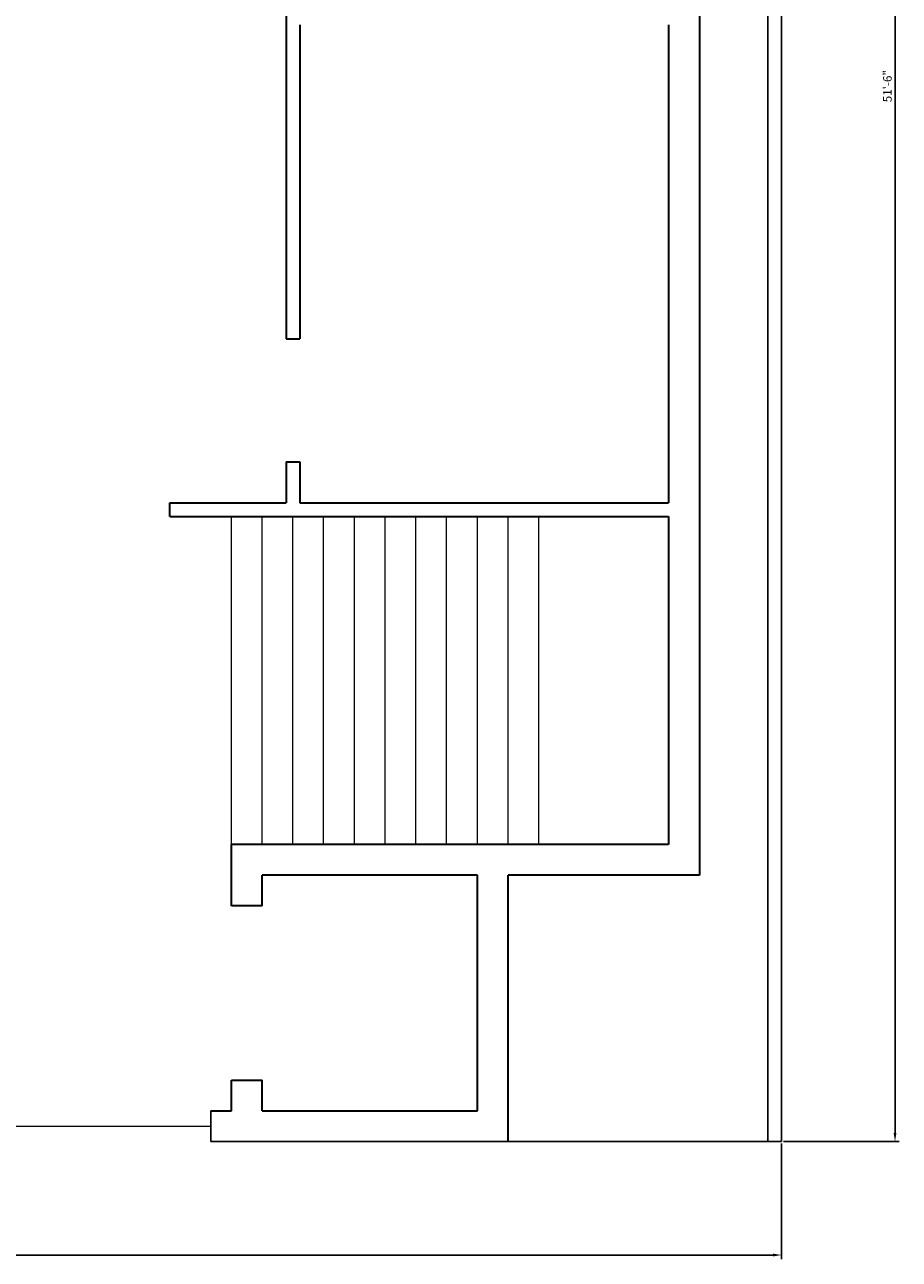
# Model space of a CAD drawing. Units: inches. Extents: x 2169 to 10664, y 1669 to 6352.
# Tile 10 of 17: x 4692 to 4948, y 1968 to 2329. Entities that reach past the tile are written whole.
import ezdxf

# ---------------------------------------------------------------- set-up
doc = ezdxf.new("R2010")
doc.units = ezdxf.units.IN
for name, color, linetype, lineweight in [('A-ANNO-DIMS', 3, 'Continuous', 18), ('A-DOOR', 4, 'Continuous', 18), ('A-FLOR-STRS', 4, 'Continuous', 18), ('A-WALL', 7, 'Continuous', 35), ('C-PROP', 251, 'Continuous', 25)]:
    doc.layers.add(name, color=color, linetype=linetype, lineweight=lineweight)
doc.styles.get("Standard").update_dxf_attribs({"font": 'arial.ttf'})
doc.dimstyles.new('ISO-25', dxfattribs={"dimtxt": 2.5, "dimasz": 2.5, "dimexe": 1.25, "dimexo": 0.625, "dimtad": 1, "dimdec": 0, "dimlunit": 3, "dimtxsty": 'Standard', "dimcen": 2.5, "dimadec": 0, "dimazin": 0, "dimtfac": 1, "dimtdec": 0, "dimtmove": 0, "dimatfit": 3, "dimfxl": 1, "dimarcsym": 0})

# ---------------------------------------------------------------- blocks, each defined once
blk = doc.blocks.new('*D102')
at = {"layer": 'A-ANNO-DIMS', "color": 0, "lineweight": -2, "transparency": 16777216}
for p, q in [((4433.57, 2001.56), (4433.57, 1967.69)), ((4913.57, 2001.56), (4913.57, 1967.69)), ((4436.07, 1968.94), (4911.07, 1968.94))]:
    blk.add_line(p, q, dxfattribs=at)
at = {"layer": 'A-ANNO-DIMS', "color": 0, "transparency": 16777216}
for points in [[(4436.07, 1969.36), (4436.07, 1968.52), (4433.57, 1968.94)], [(4911.07, 1969.36), (4911.07, 1968.52), (4913.57, 1968.94)]]:
    blk.add_solid(points, dxfattribs=at)
at = {"layer": 'Defpoints', "color": 0, "transparency": 16777216}
for p in [(4433.57, 2002.19), (4913.57, 2002.19), (4913.57, 1968.94)]:
    blk.add_point(p, dxfattribs=at)
at = {"layer": 'A-ANNO-DIMS', "color": 0, "transparency": 16777216, "insert": (4673.57, 1970.84), "char_height": 2.5, "attachment_point": 5}
blk.add_mtext('40\'-0"', dxfattribs=at)
blk = doc.blocks.new('*D103')
at = {"layer": 'A-ANNO-DIMS', "color": 0, "lineweight": -2, "transparency": 16777216}
for p, q in [((4914.2, 2620.19), (4948.07, 2620.19)), ((4946.82, 2617.69), (4946.82, 2004.69)), ((4914.2, 2002.19), (4948.07, 2002.19))]:
    blk.add_line(p, q, dxfattribs=at)
at = {"layer": 'A-ANNO-DIMS', "color": 0, "transparency": 16777216}
for points in [[(4946.41, 2617.69), (4947.24, 2617.69), (4946.82, 2620.19)], [(4946.41, 2004.69), (4947.24, 2004.69), (4946.82, 2002.19)]]:
    blk.add_solid(points, dxfattribs=at)
at = {"layer": 'Defpoints', "color": 0, "transparency": 16777216}
for p in [(4913.57, 2620.19), (4913.57, 2002.19), (4946.82, 2002.19)]:
    blk.add_point(p, dxfattribs=at)
at = {"layer": 'A-ANNO-DIMS', "color": 0, "transparency": 16777216, "insert": (4944.92, 2311.19), "char_height": 2.5, "attachment_point": 5, "rotation": 90}
blk.add_mtext('51\'-6"', dxfattribs=at)

msp = doc.modelspace()

# ---------------------------------------------------------------- linework, layer by layer
at = {"layer": 'A-DOOR'}
msp.add_line((4674.57, 2006.69), (4746.57, 2006.69), dxfattribs=at)
at = {"layer": 'A-FLOR-STRS'}
for p, q in [((4752.57, 2089.19), (4752.57, 2185.19)), ((4761.57, 2089.19), (4761.57, 2185.19)), ((4770.57, 2089.19), (4770.57, 2185.19)), ((4779.57, 2089.19), (4779.57, 2185.19)), ((4788.57, 2089.19), (4788.57, 2185.19)), ((4797.57, 2089.19), (4797.57, 2185.19)), ((4806.57, 2089.19), (4806.57, 2185.19)), ((4815.57, 2089.19), (4815.57, 2185.19)), ((4824.57, 2089.19), (4824.57, 2185.19)), ((4833.57, 2089.19), (4833.57, 2185.19)), ((4842.57, 2089.19), (4842.57, 2185.19))]:
    msp.add_line(p, q, dxfattribs=at)
at = {"layer": 'A-WALL'}
for p, q in [((4889.57, 2596.19), (4889.57, 2080.19)), ((4768.57, 2333.19), (4768.57, 2237.19)), ((4772.57, 2329.19), (4772.57, 2237.19)), ((4880.57, 2329.19), (4880.57, 2189.19)), ((4768.57, 2237.19), (4772.57, 2237.19)), ((4768.57, 2201.19), (4772.57, 2201.19)), ((4768.57, 2201.19), (4768.57, 2189.19)), ((4772.57, 2201.19), (4772.57, 2189.19)), ((4734.57, 2185.19), (4734.57, 2189.19)), ((4734.57, 2189.19), (4768.57, 2189.19)), ((4772.57, 2189.19), (4880.57, 2189.19)), ((4734.57, 2185.19), (4880.57, 2185.19)), ((4880.57, 2185.19), (4880.57, 2089.19)), ((4880.57, 2089.19), (4752.57, 2089.19)), ((4752.57, 2071.19), (4752.57, 2089.19)), ((4824.57, 2080.19), (4761.57, 2080.19)), ((4761.57, 2071.19), (4761.57, 2080.19)), ((4824.57, 2011.19), (4824.57, 2080.19)), ((4889.57, 2080.19), (4833.57, 2080.19)), ((4833.57, 2002.19), (4833.57, 2080.19)), ((4761.57, 2071.19), (4752.57, 2071.19)), ((4752.57, 2011.19), (4752.57, 2020.19)), ((4752.57, 2020.19), (4761.57, 2020.19)), ((4761.57, 2011.19), (4761.57, 2020.19)), ((4746.57, 2011.19), (4752.57, 2011.19)), ((4761.57, 2011.19), (4824.57, 2011.19))]:
    msp.add_line(p, q, dxfattribs=at)
at = {"layer": 'C-PROP'}
for p, q in [((4913.57, 2620.19), (4913.57, 2002.19)), ((4909.57, 2616.19), (4909.57, 2002.19)), ((4746.57, 2002.19), (4746.57, 2011.19)), ((4746.57, 2002.19), (4833.57, 2002.19)), ((4833.57, 2002.19), (4913.57, 2002.19))]:
    msp.add_line(p, q, dxfattribs=at)

# ---------------------------------------------------------------- dimensions: what is measured, and where the dimension line sits
at = {"layer": 'A-ANNO-DIMS'}
dim = msp.add_linear_dim(base=(4946.82, 2002.19), p1=(4913.57, 2620.19), p2=(4913.57, 2002.19), angle=90, dimstyle='ISO-25', override={"dimdec": 1, "dimlfac": 1, "dimrnd": 0, "dimzin": 1, "dimdsep": 46, "dimlunit": 4, "dimfrac": 2}, dxfattribs=at)
dim.commit()
dim.dimension.update_dxf_attribs({"geometry": '*D103', "text_midpoint": (4944.92, 2311.19)})
dim = msp.add_linear_dim(base=(4913.57, 1968.94), p1=(4433.57, 2002.19), p2=(4913.57, 2002.19), dimstyle='ISO-25', override={"dimdec": 1, "dimlfac": 1, "dimrnd": 0, "dimzin": 1, "dimdsep": 46, "dimlunit": 4, "dimfrac": 2}, dxfattribs=at)
dim.commit()
dim.dimension.update_dxf_attribs({"geometry": '*D102', "text_midpoint": (4673.57, 1970.84)})

doc.saveas('drawing.dxf')
